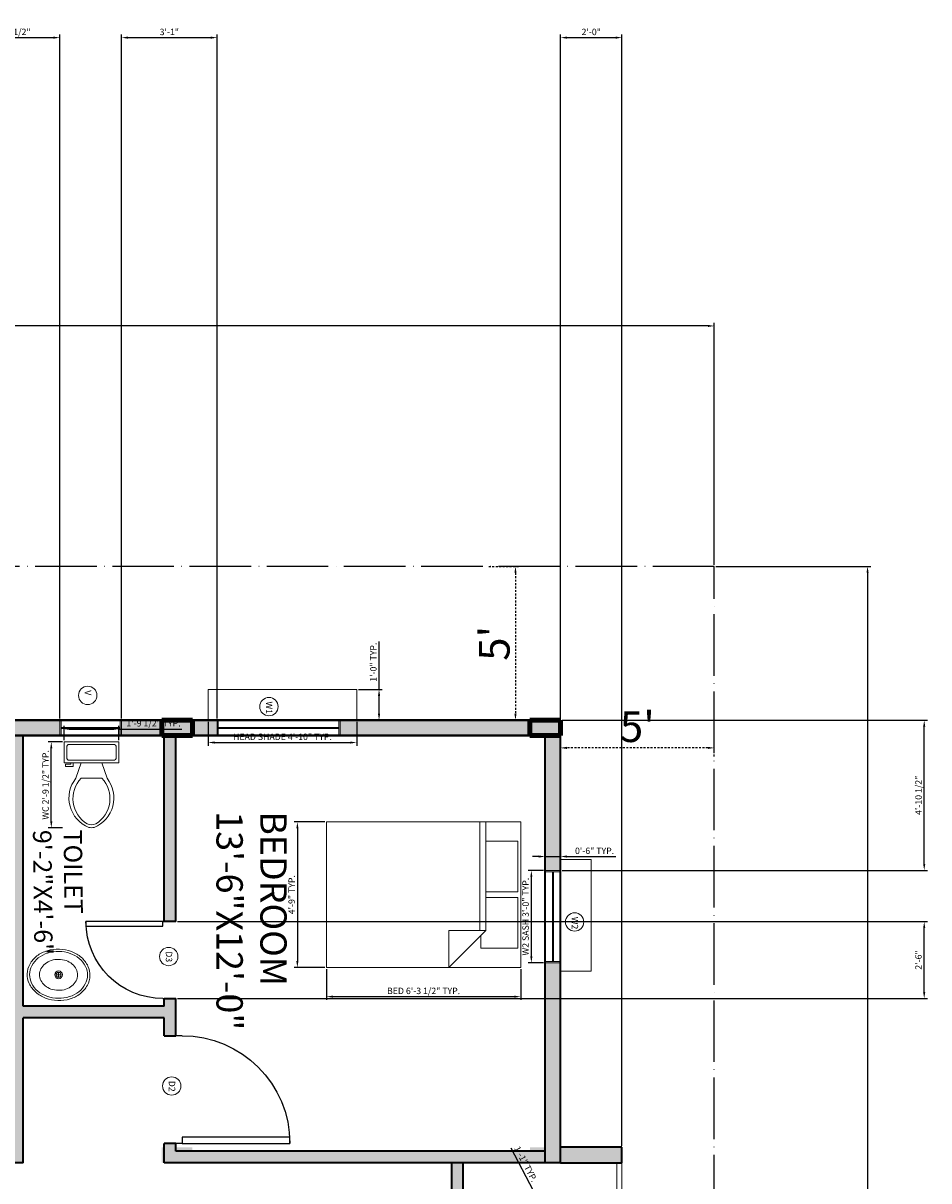
# Model space of a CAD drawing. Units: inches. Extents: x 7028582 to 7030319, y 63109697 to 63111305.
# Tile 18 of 18: x 7029966 to 7030319, y 63110853 to 63111305. Entities that reach past the tile are written whole.
import ezdxf

# ---------------------------------------------------------------- set-up
doc = ezdxf.new("R2010")
doc.units = ezdxf.units.IN
doc.linetypes.add('ACAD_ISO04W100', pattern=[30, 24, -3, 0, -3])
doc.linetypes.add('JIS_02_0.7', pattern=[1.35, 0.75, -0.6])
for name, color, linetype, lineweight in [('A-AREA-IDEN', 7, 'Continuous', 18), ('A-DOOR-IDEN', 20, 'Continuous', 13), ('A-FLOR-FIXT', 9, 'Continuous', 18), ('A-FLOR-HRAL', 5, 'Continuous', 18), ('A-GLAZ-IDEN', 20, 'Continuous', 13), ('A-WALL-PATT', 8, 'Continuous', 13), ('C-ANNO-DIMS', 7, 'Continuous', 18), ('C-PROP', 1, 'ACAD_ISO04W100', 25), ('C-STBK-DIMS', 7, 'JIS_02_0.7', 18), ('doors', 20, 'Continuous', 25), ('furniture', 9, 'Continuous', 18), ('PILLARS', 220, 'Continuous', 100), ('S-COLS-PATT', 220, 'Continuous', 100), ('walls', 6, 'Continuous', 35), ('WINDOW SHADOW', 9, 'Continuous', 13), ('windows', 5, 'Continuous', 18)]:
    doc.layers.add(name, color=color, linetype=linetype, lineweight=lineweight)
doc.styles.get("Standard").update_dxf_attribs({"font": 'arial.ttf'})
doc.dimstyles.new('ISO-25', dxfattribs={"dimtxt": 2.5, "dimasz": 2.5, "dimexe": 1.25, "dimexo": 0.625, "dimtad": 1, "dimlunit": 4, "dimtxsty": 'Standard', "dimcen": 2.5, "dimadec": 0, "dimazin": 0, "dimtfac": 1, "dimtmove": 0, "dimatfit": 3, "dimfxl": 1, "dimarcsym": 0})

# ---------------------------------------------------------------- blocks, each defined once
blk = doc.blocks.new('*U2')
for p, q in [((0, 0), (0, -5)), ((30, 0), (30, -5))]:
    blk.add_line(p, q)
blk.add_lwpolyline([(0, 0), (0, 30), (1.75, 30), (1.75, 0)], close=True)
blk.add_arc((0, 0), 30, 0, 90)
blk = doc.blocks.new('Toilet - top')
for p, q in [((9.5, -6), (9.5, -2)), ((-10, -8.5), (-8, -8.5)), ((-10, -9.5), (-10, -8.5)), ((-8, -8.5), (-8, -8)), ((-7, -8), (-7, -9.5)), ((-4, -8), (-6, -14)), ((4, -8), (6, -14)), ((-7, -9.5), (-10, -9.5)), ((4, -14), (-4, -14))]:
    blk.add_line(p, q)
blk.add_lwpolyline([(10.5, -8), (10.5, 0), (-10.5, 0), (-10.5, -8)], close=True)
for points in [[(-9.5, -2), (-9.5, -6)], [(8.5, -1), (-8.5, -1)], [(-8.5, -7), (8.5, -7)]]:
    blk.add_lwpolyline(points)
for centre, radius, start, end in [((-8.62, -1.88), 0.884, 81.8699, 188.1301), ((8.62, -1.88), 0.884, 351.8699, 98.1301), ((-8.62, -6.12), 0.884, 171.8699, 278.1301), ((8.62, -6.12), 0.884, 261.8699, 8.1301), ((3.52, -21.58), 12.17, 141.4691, 247.9714), ((4.2, -21.82), 11.33, 136.3677, 238.9468), ((-3.52, -21.58), 12.17, 292.0284, 38.5307), ((-4.2, -21.82), 11.33, 301.053, 43.6321), ((0, -27.88), 4, 245.7318, 294.2682), ((0, -29), 4, 254.8605, 285.1395)]:
    blk.add_arc(centre, radius, start, end)
blk = doc.blocks.new('Sink - Oval top')
for p, q in [((-1, 0), (1, 0)), ((0, 1), (0, -1))]:
    blk.add_line(p, q)
for points in [[(-12.23, 0.39, 0.117634), (-11.46, -3.36, 0.104469), (-8.88, -6.8, 0.090016), (-5.08, -9.07, 0.08192), (-0.32, -10.02, 0.08192), (4.49, -9.38, 0.090016), (8.42, -7.36, 0.104469), (11.22, -4.09, 0.117634), (12.23, -0.39, 0.117634), (11.46, 3.36, 0.104469), (8.88, 6.8, 0.090016), (5.08, 9.07, 0.08192), (0.32, 10.02, 0.08192), (-4.49, 9.38, 0.090016), (-8.42, 7.36, 0.104469), (-11.22, 4.09, 0.117634)], [(-11.29, 0.16, 0.118622), (-10.52, -3.25, 0.104678), (-8.07, -6.36, 0.089562), (-4.54, -8.37, 0.081185), (-0.13, -9.15, 0.081185), (4.3, -8.49, 0.089562), (7.89, -6.58, 0.104678), (10.42, -3.55, 0.118622), (11.29, -0.16, 0.118622), (10.52, 3.25, 0.104678), (8.07, 6.36, 0.089562), (4.54, 8.37, 0.081185), (0.13, 9.15, 0.081185), (-4.3, 8.49, 0.089562), (-7.89, 6.58, 0.104678), (-10.42, 3.55, 0.118622)], [(-7.42, 0.08, 0.118283), (-6.91, -2.17, 0.104607), (-5.29, -4.21, 0.089718), (-2.97, -5.53, 0.081436), (-0.07, -6.04, 0.081436), (2.84, -5.59, 0.089718), (5.2, -4.33, 0.104607), (6.86, -2.32, 0.118283), (7.42, -0.08, 0.118283), (6.91, 2.17, 0.104607), (5.29, 4.21, 0.089718), (2.97, 5.53, 0.081436), (0.07, 6.04, 0.081436), (-2.84, 5.59, 0.089718), (-5.2, 4.33, 0.104607), (-6.86, 2.32, 0.118283)]]:
    blk.add_lwpolyline(points, format="xyb", close=True)
for radius in [1.5, 1]:
    blk.add_circle((0, 0), radius)
blk = doc.blocks.new('Bed - Queen')
for p, q in [((0, -80.00003), (0, 0)), ((0, 0), (59.99999, 0)), ((59.99999, 0), (59.99999, -80.00003)), ((7.99999, -1.2), (28.79998, -1.2)), ((7.99999, -14.4), (7.99999, -1.2)), ((28.79998, -1.2), (28.79998, -14.4)), ((31.19999, -1.2), (51.99999, -1.2)), ((31.19999, -14.4), (31.19999, -1.2)), ((51.99999, -1.2), (51.99999, -16.4)), ((0, -14.4), (44.8, -14.4)), ((44.8, -16.8), (0, -16.8)), ((59.99999, -29.6), (44.8, -14.4)), ((44.8, -14.4), (44.8, -29.6)), ((51.99999, -16.4), (46.79936, -16.4)), ((44.8, -29.6), (59.99999, -29.6)), ((59.99999, -80.00003), (0, -80.00003))]:
    blk.add_line(p, q)
blk = doc.blocks.new('*D10')
at = {"layer": 'C-ANNO-DIMS', "color": 0, "lineweight": -2, "transparency": 16777216}
for p, q in [((7030236.33, 63111093.06), (7030296.71, 63111093.06)), ((7030295.46, 63111090.56), (7030295.46, 63109909.06)), ((7030236.33, 63109906.56), (7030296.71, 63109906.56))]:
    blk.add_line(p, q, dxfattribs=at)
at = {"layer": 'C-ANNO-DIMS', "color": 0, "lineweight": 100, "transparency": 16777216}
for points in [[(7030295.04, 63111090.56), (7030295.88, 63111090.56), (7030295.46, 63111093.06)], [(7030295.04, 63109909.06), (7030295.88, 63109909.06), (7030295.46, 63109906.56)]]:
    blk.add_solid(points, dxfattribs=at)
at = {"layer": 'Defpoints', "color": 0, "lineweight": 100, "transparency": 16777216}
for p in [(7030235.71, 63111093.06), (7030235.71, 63109906.56), (7030295.46, 63109906.56)]:
    blk.add_point(p, dxfattribs=at)
at = {"layer": 'C-ANNO-DIMS', "color": 0, "transparency": 16777216, "insert": (7030280.69, 63110499.81), "char_height": 12, "attachment_point": 5, "rotation": 90}
blk.add_mtext('98\'-10{\\H1x;\\S1/2;}"', dxfattribs=at)
blk = doc.blocks.new('*D11')
at = {"layer": 'C-ANNO-DIMS', "color": 0, "lineweight": -2, "transparency": 16777216}
for p, q in [((7029174.71, 63111093.68), (7029174.71, 63111188.03)), ((7030233.21, 63111186.78), (7029177.21, 63111186.78)), ((7030235.71, 63111093.68), (7030235.71, 63111188.03))]:
    blk.add_line(p, q, dxfattribs=at)
at = {"layer": 'C-ANNO-DIMS', "color": 0, "lineweight": 100, "transparency": 16777216}
for points in [[(7029177.21, 63111187.2), (7029177.21, 63111186.36), (7029174.71, 63111186.78)], [(7030233.21, 63111187.2), (7030233.21, 63111186.36), (7030235.71, 63111186.78)]]:
    blk.add_solid(points, dxfattribs=at)
at = {"layer": 'Defpoints', "color": 0, "lineweight": 100, "transparency": 16777216}
for p in [(7029174.71, 63111186.78), (7029174.71, 63111093.06), (7030235.71, 63111093.06)]:
    blk.add_point(p, dxfattribs=at)
at = {"layer": 'C-ANNO-DIMS', "color": 0, "transparency": 16777216, "insert": (7029705.21, 63111193.53), "char_height": 12, "attachment_point": 5}
blk.add_mtext('88\'-5"', dxfattribs=at)
blk = doc.blocks.new('*D12')
at = {"layer": 'C-STBK-DIMS', "color": 0, "lineweight": -2, "transparency": 16777216}
for p, q in [((7030175.71, 63111018.97), (7030175.71, 63111023.53)), ((7030235.71, 63111018.97), (7030235.71, 63111023.53)), ((7030233.21, 63111022.28), (7030178.21, 63111022.28))]:
    blk.add_line(p, q, dxfattribs=at)
at = {"layer": 'C-STBK-DIMS', "color": 0, "lineweight": 100, "transparency": 16777216}
for points in [[(7030178.21, 63111022.7), (7030178.21, 63111021.86), (7030175.71, 63111022.28)], [(7030233.21, 63111022.7), (7030233.21, 63111021.86), (7030235.71, 63111022.28)]]:
    blk.add_solid(points, dxfattribs=at)
at = {"layer": 'Defpoints', "color": 0, "lineweight": 100, "transparency": 16777216}
for p in [(7030175.71, 63111022.28), (7030175.71, 63111018.34), (7030235.71, 63111018.34)]:
    blk.add_point(p, dxfattribs=at)
at = {"layer": 'C-STBK-DIMS', "color": 0, "transparency": 16777216, "insert": (7030205.71, 63111029.01), "char_height": 12, "attachment_point": 5}
blk.add_mtext("5'", dxfattribs=at)
blk = doc.blocks.new('*D13')
at = {"layer": 'C-STBK-DIMS', "color": 0, "lineweight": -2, "transparency": 16777216}
for p, q in [((7030147.79, 63111093.06), (7030159.43, 63111093.06)), ((7030158.18, 63111090.56), (7030158.18, 63111035.56)), ((7030147.79, 63111033.06), (7030159.43, 63111033.06))]:
    blk.add_line(p, q, dxfattribs=at)
at = {"layer": 'C-STBK-DIMS', "color": 0, "lineweight": 100, "transparency": 16777216}
for points in [[(7030157.76, 63111090.56), (7030158.59, 63111090.56), (7030158.18, 63111093.06)], [(7030157.76, 63111035.56), (7030158.59, 63111035.56), (7030158.18, 63111033.06)]]:
    blk.add_solid(points, dxfattribs=at)
at = {"layer": 'Defpoints', "color": 0, "lineweight": 100, "transparency": 16777216}
for p in [(7030147.16, 63111093.06), (7030147.16, 63111033.06), (7030158.18, 63111033.06)]:
    blk.add_point(p, dxfattribs=at)
at = {"layer": 'C-STBK-DIMS', "color": 0, "transparency": 16777216, "insert": (7030151.45, 63111063.06), "char_height": 12, "attachment_point": 5, "rotation": 90}
blk.add_mtext("5'", dxfattribs=at)
blk = doc.blocks.new('WIN-SASH-36')
for p, q in [((0, 36.05), (0, 0)), ((6, 35.55), (0, 35.55)), ((2.8, 35.55), (2.8, 0.5)), ((3.2, 35.55), (3.2, 0.5)), ((6, 0), (6, 36.05)), ((0, 0.5), (6, 0.5))]:
    blk.add_line(p, q)
blk = doc.blocks.new('WIN-SASH-24')
for p, q in [((24.05, 6), (0, 6)), ((0.5, 6), (0.5, 0)), ((23.55, 0), (23.55, 6)), ((0, 0), (24.05, 0)), ((23.55, 3.2), (0.5, 3.2)), ((23.55, 2.8), (0.5, 2.8))]:
    blk.add_line(p, q)
blk = doc.blocks.new('WIN-SASH-48')
for p, q in [((48.05, 6), (0, 6)), ((0.5, 6), (0.5, 0)), ((47.55, 0), (47.55, 6)), ((47.55, 3.2), (0.5, 3.2)), ((47.55, 2.8), (0.5, 2.8)), ((0, 0), (48.05, 0))]:
    blk.add_line(p, q)
blk = doc.blocks.new('WINDOW-SHADE-SIDE-44')
for p, q in [((12, 43.55), (0, 43.55)), ((12, 0), (12, 43.55)), ((0, 0), (12, 0))]:
    blk.add_line(p, q)
blk = doc.blocks.new('WINDOW-SHADE-HEAD-58')
for p, q in [((57.96, 12), (0, 12)), ((0, 12), (0, 0)), ((57.96, 0), (57.96, 12))]:
    blk.add_line(p, q)
blk = doc.blocks.new('BALCONY-GUARD-12FT')
for p, q in [((0, 144), (0, 0)), ((2, 144), (2, 0))]:
    blk.add_line(p, q)
blk = doc.blocks.new('TAG-D2-MT-R')
blk.add_circle((3.58, 3.58), 3.58)
at = {"insert": (4.93, 5.6), "char_height": 2.5, "attachment_point": 1, "rotation": 270}
blk.add_mtext_dynamic_manual_height_columns('D2', width=2.5021, gutter_width=12.5, heights=[0], dxfattribs=at)
blk = doc.blocks.new('TAG-D3-MT-R')
blk.add_circle((3.58, 3.58), 3.58)
at = {"insert": (4.93, 5.6), "char_height": 2.5, "attachment_point": 1, "rotation": 270}
blk.add_mtext_dynamic_manual_height_columns('D3', width=2.5021, gutter_width=12.5, heights=[0], dxfattribs=at)
blk = doc.blocks.new('TAG-V-MT-R')
blk.add_circle((3.58, 3.58), 3.58)
at = {"insert": (4.93, 5.6), "char_height": 2.5, "attachment_point": 1, "rotation": 270}
blk.add_mtext_dynamic_manual_height_columns('V', width=2.5021, gutter_width=12.5, heights=[0], dxfattribs=at)
blk = doc.blocks.new('TAG-W1-MT-R')
blk.add_circle((3.58, 3.58), 3.58)
at = {"insert": (4.93, 5.6), "char_height": 2.5, "attachment_point": 1, "rotation": 270}
blk.add_mtext_dynamic_manual_height_columns('W1', width=2.5021, gutter_width=12.5, heights=[0], dxfattribs=at)
blk = doc.blocks.new('TAG-W2-MT-R')
blk.add_circle((3.58, 3.58), 3.58)
at = {"insert": (4.93, 5.6), "char_height": 2.5, "attachment_point": 1, "rotation": 270}
blk.add_mtext_dynamic_manual_height_columns('W2', width=2.5021, gutter_width=12.5, heights=[0], dxfattribs=at)
blk = doc.blocks.new('*D54')
at = {"layer": 'C-ANNO-DIMS', "color": 0, "lineweight": -2, "transparency": 16777216}
for p, q in [((7030165.17, 63110849.58), (7030156.5, 63110866.21)), ((7030163.58, 63110848.76), (7030166.27, 63110850.16)), ((7030170.13, 63110840.05), (7030166.32, 63110847.36)), ((7030169.71, 63110837.01), (7030172.4, 63110838.41))]:
    blk.add_line(p, q, dxfattribs=at)
at = {"layer": 'C-ANNO-DIMS', "color": 0, "lineweight": 100, "transparency": 16777216}
for points in [[(7030166.69, 63110847.56), (7030165.95, 63110847.17), (7030165.17, 63110849.58)], [(7030170.5, 63110840.24), (7030169.76, 63110839.86), (7030171.29, 63110837.83)]]:
    blk.add_solid(points, dxfattribs=at)
at = {"layer": 'Defpoints', "color": 0, "lineweight": 100, "transparency": 16777216}
for p in [(7030163.03, 63110848.47), (7030165.17, 63110849.58), (7030169.15, 63110836.72)]:
    blk.add_point(p, dxfattribs=at)
at = {"layer": 'C-ANNO-DIMS', "color": 0, "transparency": 16777216, "insert": (7030161.92, 63110859.87), "char_height": 2.5, "attachment_point": 5, "rotation": 297.5292}
blk.add_mtext('1\'-1" TYP.', dxfattribs=at)
blk = doc.blocks.new('*D59')
at = {"layer": 'C-ANNO-DIMS', "color": 0, "lineweight": -2, "transparency": 16777216}
for p, q in [((7029981.57, 63111024.61), (7029975.93, 63111024.61)), ((7029977.18, 63110993.61), (7029977.18, 63111022.11)), ((7029981.57, 63110991.11), (7029975.93, 63110991.11))]:
    blk.add_line(p, q, dxfattribs=at)
at = {"layer": 'C-ANNO-DIMS', "color": 0, "lineweight": 100, "transparency": 16777216}
for points in [[(7029976.76, 63111022.11), (7029977.59, 63111022.11), (7029977.18, 63111024.61)], [(7029976.76, 63110993.61), (7029977.59, 63110993.61), (7029977.18, 63110991.11)]]:
    blk.add_solid(points, dxfattribs=at)
at = {"layer": 'Defpoints', "color": 0, "lineweight": 100, "transparency": 16777216}
for p in [(7029977.18, 63111024.61), (7029982.2, 63111024.61), (7029982.2, 63110991.11)]:
    blk.add_point(p, dxfattribs=at)
at = {"layer": 'C-ANNO-DIMS', "color": 0, "transparency": 16777216, "insert": (7029975.26, 63111007.86), "char_height": 2.5, "attachment_point": 5, "rotation": 90}
blk.add_mtext('WC 2\'-9 1/2" TYP.', dxfattribs=at)
blk = doc.blocks.new('*D60')
at = {"layer": 'C-ANNO-DIMS', "color": 0, "lineweight": -2, "transparency": 16777216}
for p, q in [((7029982.2, 63111025.23), (7029982.2, 63111030.88)), ((7029984.7, 63111029.63), (7030000.98, 63111029.63)), ((7030003.48, 63111025.23), (7030003.48, 63111030.88)), ((7030003.48, 63111029.63), (7030028.06, 63111029.63))]:
    blk.add_line(p, q, dxfattribs=at)
at = {"layer": 'C-ANNO-DIMS', "color": 0, "lineweight": 100, "transparency": 16777216}
for points in [[(7029984.7, 63111030.05), (7029984.7, 63111029.21), (7029982.2, 63111029.63)], [(7030000.98, 63111030.05), (7030000.98, 63111029.21), (7030003.48, 63111029.63)]]:
    blk.add_solid(points, dxfattribs=at)
at = {"layer": 'Defpoints', "color": 0, "lineweight": 100, "transparency": 16777216}
for p in [(7030003.48, 63111029.63), (7029982.2, 63111024.61), (7030003.48, 63111024.61)]:
    blk.add_point(p, dxfattribs=at)
at = {"layer": 'C-ANNO-DIMS', "color": 0, "transparency": 16777216, "insert": (7030017.02, 63111031.55), "char_height": 2.5, "attachment_point": 5}
blk.add_mtext('1\'-9 1/2" TYP.', dxfattribs=at)
blk = doc.blocks.new('*D63')
at = {"layer": 'C-ANNO-DIMS', "color": 0, "lineweight": -2, "transparency": 16777216}
for p, q in [((7030084.49, 63110936.02), (7030084.49, 63110924.04)), ((7030160.21, 63110936.02), (7030160.21, 63110924.04)), ((7030086.99, 63110925.29), (7030157.71, 63110925.29))]:
    blk.add_line(p, q, dxfattribs=at)
at = {"layer": 'C-ANNO-DIMS', "color": 0, "lineweight": 100, "transparency": 16777216}
for points in [[(7030086.99, 63110925.71), (7030086.99, 63110924.88), (7030084.49, 63110925.29)], [(7030157.71, 63110925.71), (7030157.71, 63110924.88), (7030160.21, 63110925.29)]]:
    blk.add_solid(points, dxfattribs=at)
at = {"layer": 'Defpoints', "color": 0, "lineweight": 100, "transparency": 16777216}
for p in [(7030084.49, 63110936.65), (7030160.21, 63110936.65), (7030160.21, 63110925.29)]:
    blk.add_point(p, dxfattribs=at)
at = {"layer": 'C-ANNO-DIMS', "color": 0, "transparency": 16777216, "insert": (7030122.35, 63110927.21), "char_height": 2.5, "attachment_point": 5}
blk.add_mtext('BED 6\'-3 1/2" TYP.', dxfattribs=at)
blk = doc.blocks.new('*D64')
at = {"layer": 'C-ANNO-DIMS', "color": 0, "lineweight": -2, "transparency": 16777216}
for p, q in [((7030083.87, 63110993.43), (7030071.89, 63110993.43)), ((7030073.14, 63110990.93), (7030073.14, 63110939.15)), ((7030083.87, 63110936.65), (7030071.89, 63110936.65))]:
    blk.add_line(p, q, dxfattribs=at)
at = {"layer": 'C-ANNO-DIMS', "color": 0, "lineweight": 100, "transparency": 16777216}
for points in [[(7030072.72, 63110990.93), (7030073.55, 63110990.93), (7030073.14, 63110993.43)], [(7030072.72, 63110939.15), (7030073.55, 63110939.15), (7030073.14, 63110936.65)]]:
    blk.add_solid(points, dxfattribs=at)
at = {"layer": 'Defpoints', "color": 0, "lineweight": 100, "transparency": 16777216}
for p in [(7030084.49, 63110993.43), (7030073.14, 63110936.65), (7030084.49, 63110936.65)]:
    blk.add_point(p, dxfattribs=at)
at = {"layer": 'C-ANNO-DIMS', "color": 0, "transparency": 16777216, "insert": (7030071.23, 63110965.04), "char_height": 2.5, "attachment_point": 5, "rotation": 90}
blk.add_mtext('4\'-9" TYP.', dxfattribs=at)
blk = doc.blocks.new('*D69')
at = {"layer": 'C-ANNO-DIMS', "color": 0, "lineweight": -2, "transparency": 16777216}
for p, q in [((7030169.15, 63110974.51), (7030163.12, 63110974.51)), ((7030164.37, 63110940.97), (7030164.37, 63110972.01)), ((7030169.15, 63110938.47), (7030163.12, 63110938.47))]:
    blk.add_line(p, q, dxfattribs=at)
at = {"layer": 'C-ANNO-DIMS', "color": 0, "lineweight": 100, "transparency": 16777216}
for points in [[(7030163.95, 63110972.01), (7030164.79, 63110972.01), (7030164.37, 63110974.51)], [(7030163.95, 63110940.97), (7030164.79, 63110940.97), (7030164.37, 63110938.47)]]:
    blk.add_solid(points, dxfattribs=at)
at = {"layer": 'Defpoints', "color": 0, "lineweight": 100, "transparency": 16777216}
for p in [(7030164.37, 63110974.51), (7030169.78, 63110974.51), (7030169.78, 63110938.47)]:
    blk.add_point(p, dxfattribs=at)
at = {"layer": 'C-ANNO-DIMS', "color": 0, "transparency": 16777216, "insert": (7030162.45, 63110956.49), "char_height": 2.5, "attachment_point": 5, "rotation": 90}
blk.add_mtext('W2 SASH 3\'-0" TYP.', dxfattribs=at)
blk = doc.blocks.new('*D70')
at = {"layer": 'C-ANNO-DIMS', "color": 0, "lineweight": -2, "transparency": 16777216}
for p, q in [((7030167.28, 63110979.92), (7030164.78, 63110979.92)), ((7030169.78, 63110975.14), (7030169.78, 63110981.17)), ((7030169.78, 63110979.92), (7030175.78, 63110979.92)), ((7030175.78, 63110975.14), (7030175.78, 63110981.17)), ((7030178.28, 63110979.92), (7030197.26, 63110979.92))]:
    blk.add_line(p, q, dxfattribs=at)
at = {"layer": 'C-ANNO-DIMS', "color": 0, "lineweight": 100, "transparency": 16777216}
for points in [[(7030167.28, 63110980.34), (7030167.28, 63110979.51), (7030169.78, 63110979.92)], [(7030178.28, 63110980.34), (7030178.28, 63110979.51), (7030175.78, 63110979.92)]]:
    blk.add_solid(points, dxfattribs=at)
at = {"layer": 'Defpoints', "color": 0, "lineweight": 100, "transparency": 16777216}
for p in [(7030175.78, 63110979.92), (7030169.78, 63110974.51), (7030175.78, 63110974.51)]:
    blk.add_point(p, dxfattribs=at)
at = {"layer": 'C-ANNO-DIMS', "color": 0, "transparency": 16777216, "insert": (7030189.02, 63110981.82), "char_height": 2.5, "attachment_point": 5}
blk.add_mtext('0\'-6" TYP.', dxfattribs=at)
blk = doc.blocks.new('*D83')
at = {"layer": 'C-ANNO-DIMS', "color": 0, "lineweight": -2, "transparency": 16777216}
for p, q in [((7030038.32, 63111032.43), (7030038.32, 63111023.11)), ((7030096.29, 63111032.43), (7030096.29, 63111023.11)), ((7030040.82, 63111024.36), (7030093.79, 63111024.36))]:
    blk.add_line(p, q, dxfattribs=at)
at = {"layer": 'C-ANNO-DIMS', "color": 0, "lineweight": 100, "transparency": 16777216}
for points in [[(7030040.82, 63111024.78), (7030040.82, 63111023.95), (7030038.32, 63111024.36)], [(7030093.79, 63111024.78), (7030093.79, 63111023.95), (7030096.29, 63111024.36)]]:
    blk.add_solid(points, dxfattribs=at)
at = {"layer": 'Defpoints', "color": 0, "lineweight": 100, "transparency": 16777216}
for p in [(7030038.32, 63111033.06), (7030096.29, 63111033.06), (7030096.29, 63111024.36)]:
    blk.add_point(p, dxfattribs=at)
at = {"layer": 'C-ANNO-DIMS', "color": 0, "transparency": 16777216, "insert": (7030067.31, 63111026.28), "char_height": 2.5, "attachment_point": 5}
blk.add_mtext('HEAD SHADE 4\'-10" TYP.', dxfattribs=at)
blk = doc.blocks.new('*D84')
at = {"layer": 'C-ANNO-DIMS', "color": 0, "lineweight": -2, "transparency": 16777216}
for p, q in [((7030104.98, 63111045.06), (7030104.98, 63111063.81)), ((7030096.91, 63111045.06), (7030106.23, 63111045.06)), ((7030104.98, 63111035.56), (7030104.98, 63111042.56)), ((7030096.91, 63111033.06), (7030106.23, 63111033.06))]:
    blk.add_line(p, q, dxfattribs=at)
at = {"layer": 'C-ANNO-DIMS', "color": 0, "lineweight": 100, "transparency": 16777216}
for points in [[(7030104.57, 63111042.56), (7030105.4, 63111042.56), (7030104.98, 63111045.06)], [(7030104.57, 63111035.56), (7030105.4, 63111035.56), (7030104.98, 63111033.06)]]:
    blk.add_solid(points, dxfattribs=at)
at = {"layer": 'Defpoints', "color": 0, "lineweight": 100, "transparency": 16777216}
for p in [(7030096.29, 63111045.06), (7030104.98, 63111045.06), (7030096.29, 63111033.06)]:
    blk.add_point(p, dxfattribs=at)
at = {"layer": 'C-ANNO-DIMS', "color": 0, "transparency": 16777216, "insert": (7030103.08, 63111055.68), "char_height": 2.5, "attachment_point": 5, "rotation": 90}
blk.add_mtext('1\'-0" TYP.', dxfattribs=at)
blk = doc.blocks.new('*D101')
at = {"layer": 'C-ANNO-DIMS', "color": 0, "lineweight": -2, "transparency": 16777216}
for p, q in [((7030175.71, 63110867.18), (7030175.71, 63111300.44)), ((7030178.21, 63111299.19), (7030197.21, 63111299.19)), ((7030199.71, 63110867.18), (7030199.71, 63111300.44))]:
    blk.add_line(p, q, dxfattribs=at)
at = {"layer": 'C-ANNO-DIMS', "color": 0, "lineweight": 100, "transparency": 16777216}
for points in [[(7030178.21, 63111299.61), (7030178.21, 63111298.77), (7030175.71, 63111299.19)], [(7030197.21, 63111299.61), (7030197.21, 63111298.77), (7030199.71, 63111299.19)]]:
    blk.add_solid(points, dxfattribs=at)
at = {"layer": 'Defpoints', "color": 0, "lineweight": 100, "transparency": 16777216}
for p in [(7030199.71, 63111299.19), (7030175.71, 63110866.56), (7030199.71, 63110866.56)]:
    blk.add_point(p, dxfattribs=at)
at = {"layer": 'C-ANNO-DIMS', "color": 0, "transparency": 16777216, "insert": (7030187.71, 63111301.09), "char_height": 2.5, "attachment_point": 5}
blk.add_mtext('2\'-0"', dxfattribs=at)
blk = doc.blocks.new('*D106')
at = {"layer": 'C-ANNO-DIMS', "color": 0, "lineweight": -2, "transparency": 16777216}
for p, q in [((7030026.33, 63110954.56), (7030318.81, 63110954.56)), ((7030317.56, 63110927.06), (7030317.56, 63110952.06)), ((7030026.33, 63110924.56), (7030318.81, 63110924.56))]:
    blk.add_line(p, q, dxfattribs=at)
at = {"layer": 'C-ANNO-DIMS', "color": 0, "lineweight": 100, "transparency": 16777216}
for points in [[(7030317.14, 63110952.06), (7030317.97, 63110952.06), (7030317.56, 63110954.56)], [(7030317.14, 63110927.06), (7030317.97, 63110927.06), (7030317.56, 63110924.56)]]:
    blk.add_solid(points, dxfattribs=at)
at = {"layer": 'Defpoints', "color": 0, "lineweight": 100, "transparency": 16777216}
for p in [(7030025.71, 63110954.56), (7030317.56, 63110954.56), (7030025.71, 63110924.56)]:
    blk.add_point(p, dxfattribs=at)
at = {"layer": 'C-ANNO-DIMS', "color": 0, "transparency": 16777216, "insert": (7030315.65, 63110939.56), "char_height": 2.5, "attachment_point": 5, "rotation": 90}
blk.add_mtext('2\'-6"', dxfattribs=at)
blk = doc.blocks.new('*D115')
at = {"layer": 'C-ANNO-DIMS', "color": 0, "lineweight": -2, "transparency": 16777216}
for p, q in [((7029944.26, 63111033.68), (7029944.26, 63111300.44)), ((7029946.76, 63111299.19), (7029978.03, 63111299.19)), ((7029980.53, 63111033.68), (7029980.53, 63111300.44))]:
    blk.add_line(p, q, dxfattribs=at)
at = {"layer": 'C-ANNO-DIMS', "color": 0, "lineweight": 100, "transparency": 16777216}
for points in [[(7029946.76, 63111299.61), (7029946.76, 63111298.77), (7029944.26, 63111299.19)], [(7029978.03, 63111299.61), (7029978.03, 63111298.77), (7029980.53, 63111299.19)]]:
    blk.add_solid(points, dxfattribs=at)
at = {"layer": 'Defpoints', "color": 0, "lineweight": 100, "transparency": 16777216}
for p in [(7029980.53, 63111299.19), (7029944.26, 63111033.06), (7029980.53, 63111033.06)]:
    blk.add_point(p, dxfattribs=at)
at = {"layer": 'C-ANNO-DIMS', "color": 0, "transparency": 16777216, "insert": (7029962.39, 63111301.11), "char_height": 2.5, "attachment_point": 5}
blk.add_mtext('3\'-0 1/2"', dxfattribs=at)
blk = doc.blocks.new('*D116')
at = {"layer": 'C-ANNO-DIMS', "color": 0, "lineweight": -2, "transparency": 16777216}
for p, q in [((7030004.58, 63111033.68), (7030004.58, 63111300.44)), ((7030007.08, 63111299.19), (7030039.31, 63111299.19)), ((7030041.81, 63111033.68), (7030041.81, 63111300.44))]:
    blk.add_line(p, q, dxfattribs=at)
at = {"layer": 'C-ANNO-DIMS', "color": 0, "lineweight": 100, "transparency": 16777216}
for points in [[(7030007.08, 63111299.61), (7030007.08, 63111298.77), (7030004.58, 63111299.19)], [(7030039.31, 63111299.61), (7030039.31, 63111298.77), (7030041.81, 63111299.19)]]:
    blk.add_solid(points, dxfattribs=at)
at = {"layer": 'Defpoints', "color": 0, "lineweight": 100, "transparency": 16777216}
for p in [(7030041.81, 63111299.19), (7030004.58, 63111033.06), (7030041.81, 63111033.06)]:
    blk.add_point(p, dxfattribs=at)
at = {"layer": 'C-ANNO-DIMS', "color": 0, "transparency": 16777216, "insert": (7030023.2, 63111301.09), "char_height": 2.5, "attachment_point": 5}
blk.add_mtext('3\'-1"', dxfattribs=at)
blk = doc.blocks.new('*D117')
at = {"layer": 'C-ANNO-DIMS', "color": 0, "lineweight": -2, "transparency": 16777216}
for p, q in [((7030176.33, 63111033.06), (7030318.81, 63111033.06)), ((7030317.56, 63110977.01), (7030317.56, 63111030.56)), ((7030176.4, 63110974.51), (7030318.81, 63110974.51))]:
    blk.add_line(p, q, dxfattribs=at)
at = {"layer": 'C-ANNO-DIMS', "color": 0, "lineweight": 100, "transparency": 16777216}
for points in [[(7030317.14, 63111030.56), (7030317.97, 63111030.56), (7030317.56, 63111033.06)], [(7030317.14, 63110977.01), (7030317.97, 63110977.01), (7030317.56, 63110974.51)]]:
    blk.add_solid(points, dxfattribs=at)
at = {"layer": 'Defpoints', "color": 0, "lineweight": 100, "transparency": 16777216}
for p in [(7030175.71, 63111033.06), (7030317.56, 63111033.06), (7030175.78, 63110974.51)]:
    blk.add_point(p, dxfattribs=at)
at = {"layer": 'C-ANNO-DIMS', "color": 0, "transparency": 16777216, "insert": (7030315.64, 63111003.79), "char_height": 2.5, "attachment_point": 5, "rotation": 90}
blk.add_mtext('4\'-10 1/2"', dxfattribs=at)

msp = doc.modelspace()

# ---------------------------------------------------------------- hatches: boundary and pattern name
at = {"layer": 'A-WALL-PATT'}
h = msp.add_hatch(color=256, dxfattribs=at)
h.dxf.hatch_style = 1
h.paths.add_polyline_path([(7029980.53, 63111033.057), (7029944.258, 63111033.057), (7029944.258, 63111027.057), (7029980.53, 63111027.057)])
h = msp.add_hatch(color=256, dxfattribs=at)
h.dxf.hatch_style = 1
h.paths.add_polyline_path([(7030041.813, 63111033.057), (7030004.578, 63111033.057), (7030004.578, 63111027.057), (7030041.813, 63111027.057)])
h.paths.add_polyline_path([(7030025.705, 63111027.057), (7030021.205, 63111027.057), (7030021.205, 63110954.557), (7030025.705, 63110954.557)], flags=0)
h = msp.add_hatch(color=256, dxfattribs=at)
h.dxf.hatch_style = 1
h.paths.add_polyline_path([(7030175.705, 63111033.057), (7030089.861, 63111033.057), (7030089.861, 63111027.057), (7030169.705, 63111027.057), (7030169.705, 63110974.515), (7030175.705, 63110974.515)])
h = msp.add_hatch(color=256, dxfattribs=at)
h.dxf.hatch_style = 1
h.paths.add_polyline_path([(7030025.705, 63111027.057), (7030021.205, 63111027.057), (7030021.205, 63110954.557), (7030025.705, 63110954.557)], flags=0)
h.paths.add_polyline_path([(7030025.705, 63110924.557), (7030021.205, 63110924.557), (7030021.205, 63110921.557), (7029966.205, 63110921.557), (7029966.205, 63111027.057), (7029961.705, 63111027.057), (7029961.705, 63110921.557), (7029940.705, 63110921.557), (7029940.705, 63110917.057), (7029961.705, 63110917.057), (7029961.705, 63110865.057), (7029883.685, 63110865.057), (7029883.685, 63110860.557), (7029966.205, 63110860.557), (7029966.205, 63110917.057), (7030021.205, 63110917.057), (7030021.205, 63110910.057), (7030025.705, 63110910.057)])
h = msp.add_hatch(color=256, dxfattribs=at)
h.dxf.hatch_style = 1
h.paths.add_polyline_path([(7030025.705, 63111027.057), (7030021.205, 63111027.057), (7030021.205, 63110954.557), (7030025.705, 63110954.557)])
h = msp.add_hatch(color=256, dxfattribs=at)
h.dxf.hatch_style = 1
h.paths.add_polyline_path([(7030175.705, 63110938.466), (7030169.705, 63110938.466), (7030169.705, 63110860.557), (7030175.705, 63110860.557)])
h = msp.add_hatch(color=256, dxfattribs=at)
h.dxf.hatch_style = 1
h.paths.add_polyline_path([(7030169.705, 63110865.057), (7030025.705, 63110865.057), (7030025.705, 63110868.057), (7030021.205, 63110868.057), (7030021.205, 63110860.557), (7030169.705, 63110860.557)])
h = msp.add_hatch(color=256, dxfattribs=at)
h.dxf.hatch_style = 1
h.paths.add_polyline_path([(7030199.705, 63110866.557), (7030175.705, 63110866.557), (7030175.705, 63110860.557), (7030199.705, 63110860.557)])
h = msp.add_hatch(color=256, dxfattribs=at)
h.dxf.hatch_style = 1
h.paths.add_polyline_path([(7030137.705, 63110860.557), (7030133.205, 63110860.557), (7030133.205, 63110822.163), (7030137.705, 63110822.163)])
at = {"layer": 'S-COLS-PATT'}
h = msp.add_hatch(color=256, dxfattribs=at)
h.dxf.hatch_style = 1
h.paths.add_polyline_path([(7030032.194, 63111033.057), (7030020.279, 63111033.057), (7030020.279, 63111027.057), (7030032.194, 63111027.057)])
h = msp.add_hatch(color=256, dxfattribs=at)
h.dxf.hatch_style = 1
h.paths.add_polyline_path([(7030175.705, 63111033.057), (7030163.791, 63111033.057), (7030163.791, 63111027.057), (7030175.705, 63111027.057)])
h = msp.add_hatch(color=256, dxfattribs=at)
h.dxf.hatch_style = 1
h.paths.add_polyline_path([(7030032.194, 63110866.557), (7030020.279, 63110866.557), (7030020.279, 63110860.557), (7030032.194, 63110860.557)])
h = msp.add_hatch(color=256, dxfattribs=at)
h.dxf.hatch_style = 1
h.paths.add_polyline_path([(7030175.705, 63110866.557), (7030163.791, 63110866.557), (7030163.791, 63110860.557), (7030175.705, 63110860.557)])

# ---------------------------------------------------------------- linework, layer by layer
at = {"layer": 'C-PROP'}
for p, q in [((7030235.705, 63111093.057), (7029174.705, 63111093.057)), ((7030235.705, 63109906.557), (7030235.705, 63111093.057))]:
    msp.add_line(p, q, dxfattribs=at)
at = {"layer": 'PILLARS'}
for p, q in [((7030032.194, 63111033.057), (7030020.279, 63111033.057)), ((7030020.279, 63111033.057), (7030020.279, 63111027.057)), ((7030032.194, 63111027.057), (7030032.194, 63111033.057)), ((7030175.705, 63111033.057), (7030163.791, 63111033.057)), ((7030163.791, 63111033.057), (7030163.791, 63111027.057)), ((7030175.705, 63111027.057), (7030175.705, 63111033.057)), ((7030020.279, 63111027.057), (7030032.194, 63111027.057)), ((7030163.791, 63111027.057), (7030175.705, 63111027.057))]:
    msp.add_line(p, q, dxfattribs=at)
at = {"layer": 'walls'}
for p, q in [((7030175.705, 63111033.057), (7029234.705, 63111033.057)), ((7029234.705, 63111033.057), (7030175.705, 63111033.057)), ((7030175.705, 63110860.557), (7030175.705, 63111033.057)), ((7030169.705, 63111027.057), (7029240.705, 63111027.057)), ((7029240.705, 63111027.057), (7030169.705, 63111027.057)), ((7029966.205, 63110921.557), (7029966.205, 63111027.057)), ((7030021.205, 63110954.557), (7030021.205, 63111027.057)), ((7030025.705, 63110954.557), (7030025.705, 63111027.057)), ((7030169.705, 63110860.557), (7030169.705, 63111027.057)), ((7030025.705, 63110954.557), (7030021.205, 63110954.557)), ((7030021.205, 63110921.557), (7030021.205, 63110924.557)), ((7030021.205, 63110921.557), (7030021.205, 63110924.557)), ((7030021.205, 63110924.557), (7030025.705, 63110924.557)), ((7030025.705, 63110910.057), (7030025.705, 63110924.557)), ((7030021.205, 63110921.557), (7029966.205, 63110921.557)), ((7029966.205, 63110860.557), (7029966.205, 63110917.057)), ((7030021.205, 63110917.057), (7029966.205, 63110917.057)), ((7030021.205, 63110910.057), (7030021.205, 63110917.057)), ((7030021.205, 63110910.057), (7030025.705, 63110910.057)), ((7030021.205, 63110860.557), (7030021.205, 63110868.057)), ((7030025.705, 63110868.057), (7030021.205, 63110868.057)), ((7030025.705, 63110865.057), (7030025.705, 63110868.057)), ((7030025.705, 63110865.057), (7030025.705, 63110868.057)), ((7030169.705, 63110865.057), (7030025.705, 63110865.057)), ((7030199.705, 63110866.557), (7030175.705, 63110866.557)), ((7030199.705, 63110860.557), (7030199.705, 63110866.557)), ((7029966.205, 63110860.557), (7029883.685, 63110860.557)), ((7030175.705, 63110860.557), (7030021.205, 63110860.557)), ((7030133.205, 63110860.557), (7030133.205, 63110716.557)), ((7030137.705, 63110860.557), (7030137.705, 63110716.557)), ((7030175.705, 63110860.557), (7030199.705, 63110860.557))]:
    msp.add_line(p, q, dxfattribs=at)
at = {"layer": 'windows'}
for p, q in [((7029980.53, 63111033.057), (7029980.53, 63111027.057)), ((7030004.578, 63111027.057), (7030004.578, 63111033.057)), ((7030041.813, 63111033.057), (7030041.813, 63111027.057)), ((7030089.861, 63111027.057), (7030089.861, 63111033.057)), ((7030175.776, 63110974.515), (7030169.776, 63110974.515)), ((7030169.776, 63110938.466), (7030175.776, 63110938.466))]:
    msp.add_line(p, q, dxfattribs=at)

# ---------------------------------------------------------------- block references
at = {"layer": 'A-DOOR-IDEN'}
for name, p in [('TAG-D3-MT-R', (7030019.402, 63110937.359)), ('TAG-D2-MT-R', (7030020.567, 63110886.879))]:
    msp.add_blockref(name, p, dxfattribs=at)
at = {"layer": 'A-FLOR-FIXT', "xscale": 1.013555723357934, "yscale": 1.013555723357934, "zscale": 1.013555723357934}
msp.add_blockref('Toilet - top', (7029992.842, 63111024.605), dxfattribs=at)
at = {"layer": 'A-FLOR-FIXT'}
msp.add_blockref('Sink - Oval top', (7029980.015, 63110933.801), dxfattribs=at)
at = {"layer": 'A-FLOR-HRAL'}
msp.add_blockref('BALCONY-GUARD-12FT', (7030197.705, 63110716.557), dxfattribs=at)
at = {"layer": 'A-GLAZ-IDEN'}
for name, p in [('TAG-V-MT-R', (7029987.808, 63111039.151)), ('TAG-W1-MT-R', (7030058.467, 63111034.779)), ('TAG-W2-MT-R', (7030177.672, 63110950.827))]:
    msp.add_blockref(name, p, dxfattribs=at)
at = {"layer": 'doors', "xscale": -1, "rotation": 90}
msp.add_blockref('*U2', (7030020.705, 63110954.557), dxfattribs=at)
at = {"layer": 'doors', "xscale": -1.399999999999999, "yscale": 1.399999999999999, "zscale": 1.399999999999999, "rotation": 270}
msp.add_blockref('*U2', (7030028.205, 63110868.057), dxfattribs=at)
at = {"layer": 'furniture', "xscale": 0.9464141645025947, "yscale": 0.9464141645025947, "zscale": 0.9464141645025947, "rotation": 270}
msp.add_blockref('Bed - Queen', (7030160.206, 63110993.435), dxfattribs=at)
at = {"layer": 'WINDOW SHADOW'}
for name, p in [('WINDOW-SHADE-HEAD-58', (7030038.324, 63111033.057)), ('WINDOW-SHADE-SIDE-44', (7030175.705, 63110935.171))]:
    msp.add_blockref(name, p, dxfattribs=at)
at = {"layer": 'windows'}
for name, p in [('WIN-SASH-24', (7029980.53, 63111027.057)), ('WIN-SASH-48', (7030041.813, 63111027.057)), ('WIN-SASH-36', (7030169.776, 63110938.466))]:
    msp.add_blockref(name, p, dxfattribs=at)

# ---------------------------------------------------------------- texts
at = {"layer": 'A-AREA-IDEN', "attachment_point": 1}
for s, width, gutter_width, insert, char_height, rotation in [('BEDROOM\\P13\'-6"X12\'-0"', 82.04322, 51.315, (7030068.956, 63110997.575), 10.26307, 270), ('TOILET\\P9\'-2"X4\'-6"', 42.97461, 35.821, (7029989.133, 63110990.477), 7.16426, 270.6464)]:
    msp.add_mtext_dynamic_manual_height_columns(s, width=width, gutter_width=gutter_width, heights=[0], dxfattribs=dict(at, insert=insert, char_height=char_height, rotation=rotation))

# ---------------------------------------------------------------- dimensions: what is measured, and where the dimension line sits
at = {"layer": 'C-ANNO-DIMS'}
for base, p1, p2, override, picture, middle in [((7029980.53, 63111299.19), (7029944.258, 63111033.057), (7029980.53, 63111033.057), {"dimdec": 1, "dimlfac": 1, "dimrnd": 0, "dimzin": 1, "dimdsep": 46, "dimlunit": 4, "dimfrac": 2}, '*D115', (7029962.394, 63111301.108)), ((7030041.813, 63111299.19), (7030004.578, 63111033.057), (7030041.813, 63111033.057), {"dimdec": 1, "dimlfac": 1, "dimrnd": 0, "dimzin": 1, "dimdsep": 46, "dimlunit": 4, "dimfrac": 2}, '*D116', (7030023.196, 63111301.092)), ((7030199.705, 63111299.19), (7030175.705, 63110866.557), (7030199.705, 63110866.557), {"dimdec": 1, "dimlfac": 1, "dimrnd": 0, "dimzin": 1, "dimdsep": 46, "dimlunit": 4, "dimfrac": 2}, '*D101', (7030187.705, 63111301.091)), ((7029174.705, 63111186.781), (7030235.705, 63111093.057), (7029174.705, 63111093.057), {"dimtxt": 12, "dimclrd": 0, "dimclre": 0, "dimclrt": 0}, '*D11', (7029705.205, 63111193.533))]:
    dim = msp.add_linear_dim(base=base, p1=p1, p2=p2, dimstyle='ISO-25', override=override, dxfattribs=at)
    dim.commit()
    dim.dimension.update_dxf_attribs({"geometry": picture, "text_midpoint": middle})
for base, p1, p2, override, picture, middle in [((7030295.462, 63109906.557), (7030235.705, 63111093.057), (7030235.705, 63109906.557), {"dimtxt": 12, "dimclrd": 0, "dimclre": 0, "dimclrt": 0}, '*D10', (7030280.685, 63110499.807)), ((7030317.555, 63111033.057), (7030175.776, 63110974.515), (7030175.705, 63111033.057), {"dimdec": 1, "dimlfac": 1, "dimrnd": 0, "dimzin": 1, "dimdsep": 46, "dimlunit": 4, "dimfrac": 2}, '*D117', (7030315.638, 63111003.786)), ((7030317.555, 63110954.557), (7030025.705, 63110924.557), (7030025.705, 63110954.557), {"dimdec": 1, "dimlfac": 1, "dimrnd": 0, "dimzin": 1, "dimdsep": 46, "dimlunit": 4, "dimfrac": 2}, '*D106', (7030315.654, 63110939.557))]:
    dim = msp.add_linear_dim(base=base, p1=p1, p2=p2, angle=90, dimstyle='ISO-25', override=override, dxfattribs=at)
    dim.commit()
    dim.dimension.update_dxf_attribs({"geometry": picture, "text_midpoint": middle})
for base, p1, p2, angle, text, picture, middle in [((7030104.983, 63111045.057), (7030096.288, 63111033.057), (7030096.288, 63111045.057), 90, '<> TYP.', '*D84', (7030103.082, 63111055.683)), ((7029977.175, 63111024.605), (7029982.199, 63110991.111), (7029982.199, 63111024.605), 90, 'WC <> TYP.', '*D59', (7029975.258, 63111007.858)), ((7030073.136, 63110936.65), (7030084.493, 63110993.435), (7030084.493, 63110936.65), 270, '<> TYP.', '*D64', (7030071.235, 63110965.042)), ((7030164.369, 63110974.515), (7030169.776, 63110938.466), (7030169.776, 63110974.515), 90, 'W2 SASH <> TYP.', '*D69', (7030162.45, 63110956.49)), ((7030165.166, 63110849.58), (7030169.154, 63110836.719), (7030163.03, 63110848.468), 117.52919, '<> TYP.', '*D54', (7030161.922, 63110859.873))]:
    dim = msp.add_linear_dim(base=base, p1=p1, p2=p2, angle=angle, text=text, dimstyle='ISO-25', override={"dimdec": 1, "dimlfac": 1, "dimrnd": 0, "dimzin": 1, "dimdsep": 46, "dimlunit": 4, "dimfrac": 2}, dxfattribs=at)
    dim.commit()
    dim.dimension.update_dxf_attribs({"geometry": picture, "text_midpoint": middle})
for base, p1, p2, text, picture, middle in [((7030003.484, 63111029.63), (7029982.199, 63111024.605), (7030003.484, 63111024.605), '<> TYP.', '*D60', (7030017.023, 63111031.547)), ((7030096.288, 63111024.362), (7030038.324, 63111033.057), (7030096.288, 63111033.057), 'HEAD SHADE <> TYP.', '*D83', (7030067.306, 63111026.28)), ((7030175.776, 63110979.922), (7030169.776, 63110974.515), (7030175.776, 63110974.515), '<> TYP.', '*D70', (7030189.02, 63110981.823)), ((7030160.206, 63110925.293), (7030084.493, 63110936.65), (7030160.206, 63110936.65), 'BED <> TYP.', '*D63', (7030122.35, 63110927.211))]:
    dim = msp.add_linear_dim(base=base, p1=p1, p2=p2, text=text, dimstyle='ISO-25', override={"dimdec": 1, "dimlfac": 1, "dimrnd": 0, "dimzin": 1, "dimdsep": 46, "dimlunit": 4, "dimfrac": 2}, dxfattribs=at)
    dim.commit()
    dim.dimension.update_dxf_attribs({"geometry": picture, "text_midpoint": middle})
at = {"layer": 'C-STBK-DIMS'}
dim = msp.add_linear_dim(base=(7030158.178, 63111033.057), p1=(7030147.161, 63111093.057), p2=(7030147.161, 63111033.057), angle=90, dimstyle='ISO-25', override={"dimtxt": 12, "dimclrd": 0, "dimclre": 0, "dimclrt": 0}, dxfattribs=at)
dim.commit()
dim.dimension.update_dxf_attribs({"geometry": '*D13', "text_midpoint": (7030151.45, 63111063.057)})
dim = msp.add_linear_dim(base=(7030175.705, 63111022.279), p1=(7030235.705, 63111018.342), p2=(7030175.705, 63111018.342), dimstyle='ISO-25', override={"dimtxt": 12, "dimclrd": 0, "dimclre": 0, "dimclrt": 0}, dxfattribs=at)
dim.commit()
dim.dimension.update_dxf_attribs({"geometry": '*D12', "text_midpoint": (7030205.705, 63111029.007)})

doc.saveas('drawing.dxf')
